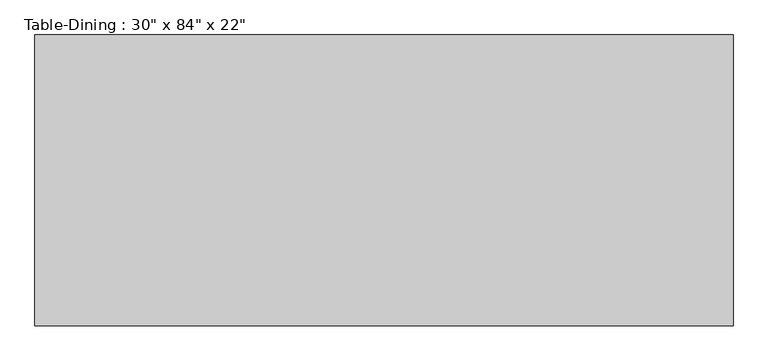
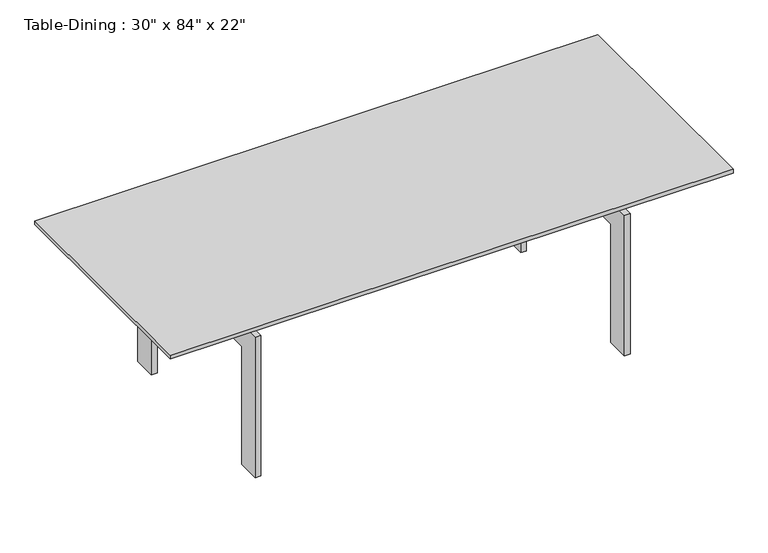
"""IFC4 building model written with IfcOpenShell, lengths in millimetres: furniture geometry."""

from ifc_helpers import new_model, si_unit, frame, origin, place, context, project, spatial, polyline, outline, extrude, source, transform, mapped, element, save


def furniture_c1c323c4(model_context):
    return source(origin(), model_context, "Body", "SweptSolid", [
        extrude(outline(polyline([(831.0657667, 297.7823857), (831.0657667, 272.3823857), (-794.5342333, 272.3823857), (-794.5342333, 297.7823857), (831.0657667, 297.7823857)])), frame((0.0, 0.0, 482.6), z_axis=(0.0, 0.0, 1.0), x_axis=(1.0, 0.0, 0.0)), (0.0, 0.0, 1.0), 63.5),
        extrude(outline(polyline([(831.0657667, -82.5889222), (831.0657667, -107.9889222), (-794.5342333, -107.9889222), (-794.5342333, -82.5889222), (831.0657667, -82.5889222)])), frame((0.0, 0.0, 482.6), z_axis=(0.0, 0.0, 1.0), x_axis=(1.0, 0.0, 0.0)), (0.0, 0.0, 1.0), 63.5),
        extrude(outline(polyline([(425.4110778, 0.0), (349.2110778, 0.0), (349.2110778, 406.4), (-158.7889222, 406.4), (-158.7889222, 0.0), (-234.9889222, 0.0), (-234.9889222, 482.6), (425.4110778, 482.6), (425.4110778, 0.0)])), frame((608.8157667, 0.0, 0.0), z_axis=(1.0, 0.0, 0.0), x_axis=(0.0, 1.0, 0.0)), (0.0, 0.0, 1.0), 19.05),
        extrude(outline(polyline([(425.4110778, 482.6), (425.4110778, 0.0), (349.2110778, 0.0), (349.2110778, 406.4), (-158.7889222, 406.4), (-158.7889222, 0.0), (-234.9889222, 0.0), (-234.9889222, 482.6), (425.4110778, 482.6)])), frame((-591.3342333, 0.0, 0.0), z_axis=(1.0, 0.0, 0.0), x_axis=(0.0, 1.0, 0.0)), (0.0, 0.0, 1.0), 19.05),
        extrude(outline(polyline([(932.6657667, 476.2110778), (932.6657667, -285.7889222), (-896.1342333, -285.7889222), (-896.1342333, 476.2110778), (932.6657667, 476.2110778)])), frame((0.0, 0.0, 546.1), z_axis=(0.0, 0.0, 1.0), x_axis=(1.0, 0.0, 0.0)), (0.0, 0.0, 1.0), 12.7),
    ])


if __name__ == "__main__":
    model = new_model("IFC4")
    model_context = context("Model", 3, world=origin())
    ifc_project = project(units=[si_unit("LENGTHUNIT", "METRE", prefix="MILLI")], contexts=[model_context])
    site = spatial("IfcSite", under=ifc_project)
    building = spatial("IfcBuilding", under=site)
    placement = place(None, origin())
    furniture_shape = furniture_c1c323c4(model_context)
    element("IfcFurniture", 1, ObjectType="Table-Dining : 30\" x 84\" x 22\"", at=placement, inside=building, context=model_context, shape_type="MappedRepresentation", body=[
        mapped(furniture_shape, transform((0.0, 0.0, 0.0), x_axis=(1.0, 0.0, 0.0), y_axis=(0.0, 1.0, 0.0), z_axis=(0.0, 0.0, 1.0))),
    ])
    save(model, "model.ifc")

# Revit data of these elements
# Type "Table-Dining : 30\" x 84\" x 22\""
#   Assembly Code = "E2020200"
#   Height = 1' - 10"
#   Length = 6' - 0"
#   Width = 2' - 6"
#   Base Material = Steel, Chrome Plated
#   Top Material = Glass - Clear, Grey
#   Default Elevation = 0
# Element 1 (IfcFurniture, "Table-Dining : 30\" x 84\" x 22\"")
#   Materials on its faces: "Steel, Chrome Plated", "Glass - Clear, Grey"
# Materials
#   "Steel, Chrome Plated": class "Metal", colour RGB 17 17 17, transparency 0, Description = "Chromiuim plated steel", Cost = 0
#   "Glass - Clear, Grey": class "Glass", colour RGB 252 255 255, transparency 0.64
